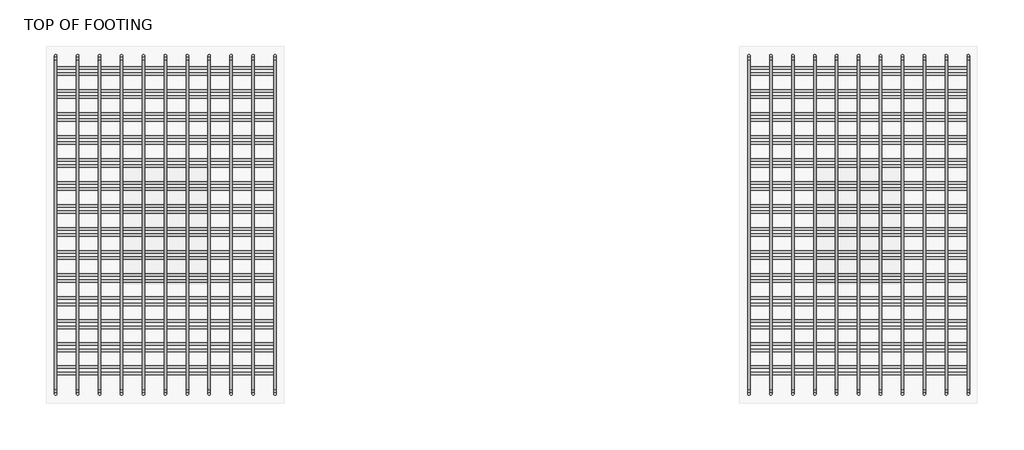
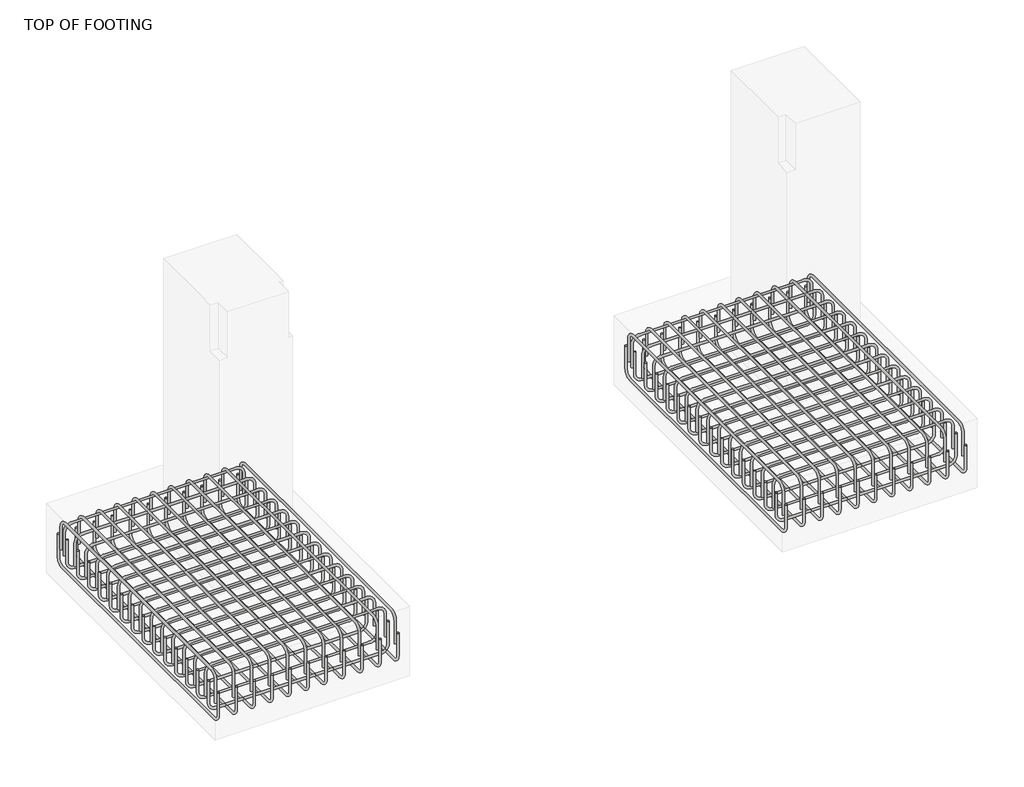
# One storey, part 11 of 11: 8 reinforcing bars.
"""IFC4 building model written with IfcOpenShell, lengths in millimetres."""

from ifc_helpers import new_model, si_unit, point, frame, origin, place, context, project, spatial, polyline, circle_curve, trimmed, segment, composite_curve, source, transform, mapped, element, save
from ifc_brep_helpers import swept_disk

model = new_model("IFC4")

# Units and contexts
model_context = context("Model", 3, world=origin())
ifc_project = project(units=[si_unit("LENGTHUNIT", "METRE", prefix="MILLI")], contexts=[model_context])

# Site, building, storey
site = spatial("IfcSite", under=ifc_project)
building = spatial("IfcBuilding", under=site)
storey = spatial("IfcBuildingStorey", under=building, Name="TOP OF FOOTING", Elevation=-1828.8)

# Reinforcing bars
placement = place(None, origin())
reinforcing_bar_shape = source(origin(), model_context, "Body", "SolidModel", [
    swept_disk(composite_curve([segment(polyline([(5183.7615906, 18549.4712443, -2012.1658531), (5183.7615906, 18549.4712443, -2159.4658531)]), True, "CONTINUOUS"), segment(trimmed(circle_curve(frame((5183.7615906, 18595.8212443, -2159.4658531), z_axis=(1.0, 0.0, 0.0), x_axis=(0.0, -46.35000000000218, 0.0)), 46.35), [point((5183.7615906, 18549.4712443, -2159.4658531))], [point((5183.7615906, 18595.8212443, -2205.8158531))], True, "CARTESIAN"), True, "CONTINUOUS"), segment(polyline([(5183.7615906, 18595.8212443, -2205.8158531), (5183.7615906, 20210.4212443, -2205.8158531)]), True, "CONTINUOUS"), segment(trimmed(circle_curve(frame((5183.7615906, 20210.4212443, -2159.4658531), z_axis=(1.0, 0.0, 0.0), x_axis=(0.0, 0.0, -46.34999999999991)), 46.35), [point((5183.7615906, 20210.4212443, -2205.8158531))], [point((5183.7615906, 20256.7712443, -2159.4658531))], True, "CARTESIAN"), True, "CONTINUOUS"), segment(polyline([(5183.7615906, 20256.7712443, -2159.4658531), (5183.7615906, 20256.7712443, -2012.1658531)]), True, "CONTINUOUS")], self_intersect=False), 6.35),
])
element("IfcReinforcingBar", 1, at=placement, inside=storey, context=model_context, shape_type="MappedRepresentation", body=[
    mapped(reinforcing_bar_shape, transform((0.0, 0.0, 0.0), x_axis=(1.0, 0.0, 0.0), y_axis=(0.0, 1.0, 0.0), z_axis=(0.0, 0.0, 1.0))),
    mapped(reinforcing_bar_shape, transform((-110.73, 0.0, 0.0), x_axis=(1.0, 0.0, 0.0), y_axis=(0.0, 1.0, 0.0), z_axis=(0.0, 0.0, 1.0))),
    mapped(reinforcing_bar_shape, transform((-221.46, 0.0, 0.0), x_axis=(1.0, 0.0, 0.0), y_axis=(0.0, 1.0, 0.0), z_axis=(0.0, 0.0, 1.0))),
    mapped(reinforcing_bar_shape, transform((-332.19, 0.0, 0.0), x_axis=(1.0, 0.0, 0.0), y_axis=(0.0, 1.0, 0.0), z_axis=(0.0, 0.0, 1.0))),
    mapped(reinforcing_bar_shape, transform((-442.92, 0.0, 0.0), x_axis=(1.0, 0.0, 0.0), y_axis=(0.0, 1.0, 0.0), z_axis=(0.0, 0.0, 1.0))),
    mapped(reinforcing_bar_shape, transform((-553.65, 0.0, 0.0), x_axis=(1.0, 0.0, 0.0), y_axis=(0.0, 1.0, 0.0), z_axis=(0.0, 0.0, 1.0))),
    mapped(reinforcing_bar_shape, transform((-664.38, 0.0, 0.0), x_axis=(1.0, 0.0, 0.0), y_axis=(0.0, 1.0, 0.0), z_axis=(0.0, 0.0, 1.0))),
    mapped(reinforcing_bar_shape, transform((-775.11, 0.0, 0.0), x_axis=(1.0, 0.0, 0.0), y_axis=(0.0, 1.0, 0.0), z_axis=(0.0, 0.0, 1.0))),
    mapped(reinforcing_bar_shape, transform((-885.84, 0.0, 0.0), x_axis=(1.0, 0.0, 0.0), y_axis=(0.0, 1.0, 0.0), z_axis=(0.0, 0.0, 1.0))),
    mapped(reinforcing_bar_shape, transform((-996.57, 0.0, 0.0), x_axis=(1.0, 0.0, 0.0), y_axis=(0.0, 1.0, 0.0), z_axis=(0.0, 0.0, 1.0))),
    mapped(reinforcing_bar_shape, transform((-1107.3, 0.0, 0.0), x_axis=(1.0, 0.0, 0.0), y_axis=(0.0, 1.0, 0.0), z_axis=(0.0, 0.0, 1.0))),
])
reinforcing_bar_2_shape = source(origin(), model_context, "Body", "SolidModel", [
    swept_disk(composite_curve([segment(polyline([(4076.4615906, 18577.6603603, -2096.8914539), (4076.4615906, 18577.6603603, -1949.5914539)]), True, "CONTINUOUS"), segment(trimmed(circle_curve(frame((4076.4615906, 18624.0103603, -1949.5914539), z_axis=(-1.0, 0.0, 0.0), x_axis=(0.0, -46.349999999998545, 0.0)), 46.35), [point((4076.4615906, 18577.6603603, -1949.5914539))], [point((4076.4615906, 18624.0103603, -1903.2414539))], True, "CARTESIAN"), True, "CONTINUOUS"), segment(polyline([(4076.4615906, 18624.0103603, -1903.2414539), (4076.4615906, 20181.3238837, -1903.2414539)]), True, "CONTINUOUS"), segment(trimmed(circle_curve(frame((4076.4615906, 20181.3238837, -1949.5914539), z_axis=(-1.0, 0.0, 0.0), x_axis=(0.0, 0.0, 46.350000000000136)), 46.35), [point((4076.4615906, 20181.3238837, -1903.2414539))], [point((4076.4615906, 20227.6738837, -1949.5914539))], True, "CARTESIAN"), True, "CONTINUOUS"), segment(polyline([(4076.4615906, 20227.6738837, -1949.5914539), (4076.4615906, 20227.6738837, -2096.8914539)]), True, "CONTINUOUS")], self_intersect=False), 6.35),
])
element("IfcReinforcingBar", 2, at=placement, inside=storey, context=model_context, shape_type="MappedRepresentation", body=[
    mapped(reinforcing_bar_2_shape, transform((0.0, 0.0, 0.0), x_axis=(1.0, 0.0, 0.0), y_axis=(0.0, 1.0, 0.0), z_axis=(0.0, 0.0, 1.0))),
    mapped(reinforcing_bar_2_shape, transform((110.73, 0.0, 0.0), x_axis=(1.0, 0.0, 0.0), y_axis=(0.0, 1.0, 0.0), z_axis=(0.0, 0.0, 1.0))),
    mapped(reinforcing_bar_2_shape, transform((221.46, 0.0, 0.0), x_axis=(1.0, 0.0, 0.0), y_axis=(0.0, 1.0, 0.0), z_axis=(0.0, 0.0, 1.0))),
    mapped(reinforcing_bar_2_shape, transform((332.19, 0.0, 0.0), x_axis=(1.0, 0.0, 0.0), y_axis=(0.0, 1.0, 0.0), z_axis=(0.0, 0.0, 1.0))),
    mapped(reinforcing_bar_2_shape, transform((442.92, 0.0, 0.0), x_axis=(1.0, 0.0, 0.0), y_axis=(0.0, 1.0, 0.0), z_axis=(0.0, 0.0, 1.0))),
    mapped(reinforcing_bar_2_shape, transform((553.65, 0.0, 0.0), x_axis=(1.0, 0.0, 0.0), y_axis=(0.0, 1.0, 0.0), z_axis=(0.0, 0.0, 1.0))),
    mapped(reinforcing_bar_2_shape, transform((664.38, 0.0, 0.0), x_axis=(1.0, 0.0, 0.0), y_axis=(0.0, 1.0, 0.0), z_axis=(0.0, 0.0, 1.0))),
    mapped(reinforcing_bar_2_shape, transform((775.11, 0.0, 0.0), x_axis=(1.0, 0.0, 0.0), y_axis=(0.0, 1.0, 0.0), z_axis=(0.0, 0.0, 1.0))),
    mapped(reinforcing_bar_2_shape, transform((885.84, 0.0, 0.0), x_axis=(1.0, 0.0, 0.0), y_axis=(0.0, 1.0, 0.0), z_axis=(0.0, 0.0, 1.0))),
    mapped(reinforcing_bar_2_shape, transform((996.57, 0.0, 0.0), x_axis=(1.0, 0.0, 0.0), y_axis=(0.0, 1.0, 0.0), z_axis=(0.0, 0.0, 1.0))),
    mapped(reinforcing_bar_2_shape, transform((1107.3, 0.0, 0.0), x_axis=(1.0, 0.0, 0.0), y_axis=(0.0, 1.0, 0.0), z_axis=(0.0, 0.0, 1.0))),
])
reinforcing_bar_3_shape = source(origin(), model_context, "Body", "SolidModel", [
    swept_disk(composite_curve([segment(polyline([(4076.4615906, 18653.1930221, -1996.7664426), (4076.4615906, 18653.1930221, -2144.0664426)]), True, "CONTINUOUS"), segment(trimmed(circle_curve(frame((4122.8115906, 18653.1930221, -2144.0664426), z_axis=(0.0, -1.0, 0.0), x_axis=(-46.350000000000364, 0.0, 0.0)), 46.35), [point((4076.4615906, 18653.1930221, -2144.0664426))], [point((4122.8115906, 18653.1930221, -2190.4164426))], True, "CARTESIAN"), True, "CONTINUOUS"), segment(polyline([(4122.8115906, 18653.1930221, -2190.4164426), (5137.4115906, 18653.1930221, -2190.4164426)]), True, "CONTINUOUS"), segment(trimmed(circle_curve(frame((5137.4115906, 18653.1930221, -2144.0664426), z_axis=(0.0, -1.0, 0.0), x_axis=(0.0, 0.0, -46.350000000000364)), 46.35), [point((5137.4115906, 18653.1930221, -2190.4164426))], [point((5183.7615906, 18653.1930221, -2144.0664426))], True, "CARTESIAN"), True, "CONTINUOUS"), segment(polyline([(5183.7615906, 18653.1930221, -2144.0664426), (5183.7615906, 18653.1930221, -1996.7664426)]), True, "CONTINUOUS")], self_intersect=False), 6.35),
])
element("IfcReinforcingBar", 3, at=placement, inside=storey, context=model_context, shape_type="MappedRepresentation", body=[
    mapped(reinforcing_bar_3_shape, transform((0.0, 0.0, 0.0), x_axis=(1.0, 0.0, 0.0), y_axis=(0.0, 1.0, 0.0), z_axis=(0.0, 0.0, 1.0))),
    mapped(reinforcing_bar_3_shape, transform((0.0, 116.2744005, 0.0), x_axis=(1.0, 0.0, 0.0), y_axis=(0.0, 1.0, 0.0), z_axis=(0.0, 0.0, 1.0))),
    mapped(reinforcing_bar_3_shape, transform((0.0, 232.5488009, 0.0), x_axis=(1.0, 0.0, 0.0), y_axis=(0.0, 1.0, 0.0), z_axis=(0.0, 0.0, 1.0))),
    mapped(reinforcing_bar_3_shape, transform((0.0, 348.8232014, 0.0), x_axis=(1.0, 0.0, 0.0), y_axis=(0.0, 1.0, 0.0), z_axis=(0.0, 0.0, 1.0))),
    mapped(reinforcing_bar_3_shape, transform((0.0, 465.0976018, 0.0), x_axis=(1.0, 0.0, 0.0), y_axis=(0.0, 1.0, 0.0), z_axis=(0.0, 0.0, 1.0))),
    mapped(reinforcing_bar_3_shape, transform((0.0, 581.3720023, 0.0), x_axis=(1.0, 0.0, 0.0), y_axis=(0.0, 1.0, 0.0), z_axis=(0.0, 0.0, 1.0))),
    mapped(reinforcing_bar_3_shape, transform((0.0, 697.6464027, 0.0), x_axis=(1.0, 0.0, 0.0), y_axis=(0.0, 1.0, 0.0), z_axis=(0.0, 0.0, 1.0))),
    mapped(reinforcing_bar_3_shape, transform((0.0, 813.9208032, 0.0), x_axis=(1.0, 0.0, 0.0), y_axis=(0.0, 1.0, 0.0), z_axis=(0.0, 0.0, 1.0))),
    mapped(reinforcing_bar_3_shape, transform((0.0, 930.1952036, 0.0), x_axis=(1.0, 0.0, 0.0), y_axis=(0.0, 1.0, 0.0), z_axis=(0.0, 0.0, 1.0))),
    mapped(reinforcing_bar_3_shape, transform((0.0, 1046.4696041, 0.0), x_axis=(1.0, 0.0, 0.0), y_axis=(0.0, 1.0, 0.0), z_axis=(0.0, 0.0, 1.0))),
    mapped(reinforcing_bar_3_shape, transform((0.0, 1162.7440045, 0.0), x_axis=(1.0, 0.0, 0.0), y_axis=(0.0, 1.0, 0.0), z_axis=(0.0, 0.0, 1.0))),
    mapped(reinforcing_bar_3_shape, transform((0.0, 1279.018405, 0.0), x_axis=(1.0, 0.0, 0.0), y_axis=(0.0, 1.0, 0.0), z_axis=(0.0, 0.0, 1.0))),
    mapped(reinforcing_bar_3_shape, transform((0.0, 1395.2928054, 0.0), x_axis=(1.0, 0.0, 0.0), y_axis=(0.0, 1.0, 0.0), z_axis=(0.0, 0.0, 1.0))),
    mapped(reinforcing_bar_3_shape, transform((0.0, 1511.5672059, 0.0), x_axis=(1.0, 0.0, 0.0), y_axis=(0.0, 1.0, 0.0), z_axis=(0.0, 0.0, 1.0))),
])
reinforcing_bar_4_shape = source(origin(), model_context, "Body", "SolidModel", [
    swept_disk(composite_curve([segment(polyline([(4076.4615906, 20194.4257435, -2114.1958609), (4076.4615906, 20194.4257435, -1966.8958609)]), True, "CONTINUOUS"), segment(trimmed(circle_curve(frame((4122.8115906, 20194.4257435, -1966.8958609), z_axis=(0.0, 1.0, 0.0), x_axis=(-46.350000000000364, 0.0, 0.0)), 46.35), [point((4076.4615906, 20194.4257435, -1966.8958609))], [point((4122.8115906, 20194.4257435, -1920.5458609))], True, "CARTESIAN"), True, "CONTINUOUS"), segment(polyline([(4122.8115906, 20194.4257435, -1920.5458609), (5137.4115906, 20194.4257435, -1920.5458609)]), True, "CONTINUOUS"), segment(trimmed(circle_curve(frame((5137.4115906, 20194.4257435, -1966.8958609), z_axis=(0.0, 1.0, 0.0), x_axis=(0.0, 0.0, 46.34999999999991)), 46.35), [point((5137.4115906, 20194.4257435, -1920.5458609))], [point((5183.7615906, 20194.4257435, -1966.8958609))], True, "CARTESIAN"), True, "CONTINUOUS"), segment(polyline([(5183.7615906, 20194.4257435, -1966.8958609), (5183.7615906, 20194.4257435, -2114.1958609)]), True, "CONTINUOUS")], self_intersect=False), 6.35),
])
element("IfcReinforcingBar", 4, at=placement, inside=storey, context=model_context, shape_type="MappedRepresentation", body=[
    mapped(reinforcing_bar_4_shape, transform((0.0, 0.0, 0.0), x_axis=(1.0, 0.0, 0.0), y_axis=(0.0, 1.0, 0.0), z_axis=(0.0, 0.0, 1.0))),
    mapped(reinforcing_bar_4_shape, transform((0.0, -116.1057918, 0.0), x_axis=(1.0, 0.0, 0.0), y_axis=(0.0, 1.0, 0.0), z_axis=(0.0, 0.0, 1.0))),
    mapped(reinforcing_bar_4_shape, transform((0.0, -232.2115836, 0.0), x_axis=(1.0, 0.0, 0.0), y_axis=(0.0, 1.0, 0.0), z_axis=(0.0, 0.0, 1.0))),
    mapped(reinforcing_bar_4_shape, transform((0.0, -348.3173754, 0.0), x_axis=(1.0, 0.0, 0.0), y_axis=(0.0, 1.0, 0.0), z_axis=(0.0, 0.0, 1.0))),
    mapped(reinforcing_bar_4_shape, transform((0.0, -464.4231672, 0.0), x_axis=(1.0, 0.0, 0.0), y_axis=(0.0, 1.0, 0.0), z_axis=(0.0, 0.0, 1.0))),
    mapped(reinforcing_bar_4_shape, transform((0.0, -580.528959, 0.0), x_axis=(1.0, 0.0, 0.0), y_axis=(0.0, 1.0, 0.0), z_axis=(0.0, 0.0, 1.0))),
    mapped(reinforcing_bar_4_shape, transform((0.0, -696.6347508, 0.0), x_axis=(1.0, 0.0, 0.0), y_axis=(0.0, 1.0, 0.0), z_axis=(0.0, 0.0, 1.0))),
    mapped(reinforcing_bar_4_shape, transform((0.0, -812.7405426, 0.0), x_axis=(1.0, 0.0, 0.0), y_axis=(0.0, 1.0, 0.0), z_axis=(0.0, 0.0, 1.0))),
    mapped(reinforcing_bar_4_shape, transform((0.0, -928.8463344, 0.0), x_axis=(1.0, 0.0, 0.0), y_axis=(0.0, 1.0, 0.0), z_axis=(0.0, 0.0, 1.0))),
    mapped(reinforcing_bar_4_shape, transform((0.0, -1044.9521262, 0.0), x_axis=(1.0, 0.0, 0.0), y_axis=(0.0, 1.0, 0.0), z_axis=(0.0, 0.0, 1.0))),
    mapped(reinforcing_bar_4_shape, transform((0.0, -1161.057918, 0.0), x_axis=(1.0, 0.0, 0.0), y_axis=(0.0, 1.0, 0.0), z_axis=(0.0, 0.0, 1.0))),
    mapped(reinforcing_bar_4_shape, transform((0.0, -1277.1637098, 0.0), x_axis=(1.0, 0.0, 0.0), y_axis=(0.0, 1.0, 0.0), z_axis=(0.0, 0.0, 1.0))),
    mapped(reinforcing_bar_4_shape, transform((0.0, -1393.2695016, 0.0), x_axis=(1.0, 0.0, 0.0), y_axis=(0.0, 1.0, 0.0), z_axis=(0.0, 0.0, 1.0))),
    mapped(reinforcing_bar_4_shape, transform((0.0, -1509.3752934, 0.0), x_axis=(1.0, 0.0, 0.0), y_axis=(0.0, 1.0, 0.0), z_axis=(0.0, 0.0, 1.0))),
])
reinforcing_bar_5_shape = source(origin(), model_context, "Body", "SolidModel", [
    swept_disk(composite_curve([segment(polyline([(8683.7615906, 18549.4712443, -2012.1658531), (8683.7615906, 18549.4712443, -2159.4658531)]), True, "CONTINUOUS"), segment(trimmed(circle_curve(frame((8683.7615906, 18595.8212443, -2159.4658531), z_axis=(1.0, 0.0, 0.0), x_axis=(0.0, -46.35000000000218, 0.0)), 46.35), [point((8683.7615906, 18549.4712443, -2159.4658531))], [point((8683.7615906, 18595.8212443, -2205.8158531))], True, "CARTESIAN"), True, "CONTINUOUS"), segment(polyline([(8683.7615906, 18595.8212443, -2205.8158531), (8683.7615906, 20210.4212443, -2205.8158531)]), True, "CONTINUOUS"), segment(trimmed(circle_curve(frame((8683.7615906, 20210.4212443, -2159.4658531), z_axis=(1.0, 0.0, 0.0), x_axis=(0.0, 0.0, -46.34999999999991)), 46.35), [point((8683.7615906, 20210.4212443, -2205.8158531))], [point((8683.7615906, 20256.7712443, -2159.4658531))], True, "CARTESIAN"), True, "CONTINUOUS"), segment(polyline([(8683.7615906, 20256.7712443, -2159.4658531), (8683.7615906, 20256.7712443, -2012.1658531)]), True, "CONTINUOUS")], self_intersect=False), 6.35),
])
element("IfcReinforcingBar", 5, at=placement, inside=storey, context=model_context, shape_type="MappedRepresentation", body=[
    mapped(reinforcing_bar_5_shape, transform((0.0, 0.0, 0.0), x_axis=(1.0, 0.0, 0.0), y_axis=(0.0, 1.0, 0.0), z_axis=(0.0, 0.0, 1.0))),
    mapped(reinforcing_bar_5_shape, transform((-110.73, 0.0, 0.0), x_axis=(1.0, 0.0, 0.0), y_axis=(0.0, 1.0, 0.0), z_axis=(0.0, 0.0, 1.0))),
    mapped(reinforcing_bar_5_shape, transform((-221.46, 0.0, 0.0), x_axis=(1.0, 0.0, 0.0), y_axis=(0.0, 1.0, 0.0), z_axis=(0.0, 0.0, 1.0))),
    mapped(reinforcing_bar_5_shape, transform((-332.19, 0.0, 0.0), x_axis=(1.0, 0.0, 0.0), y_axis=(0.0, 1.0, 0.0), z_axis=(0.0, 0.0, 1.0))),
    mapped(reinforcing_bar_5_shape, transform((-442.92, 0.0, 0.0), x_axis=(1.0, 0.0, 0.0), y_axis=(0.0, 1.0, 0.0), z_axis=(0.0, 0.0, 1.0))),
    mapped(reinforcing_bar_5_shape, transform((-553.65, 0.0, 0.0), x_axis=(1.0, 0.0, 0.0), y_axis=(0.0, 1.0, 0.0), z_axis=(0.0, 0.0, 1.0))),
    mapped(reinforcing_bar_5_shape, transform((-664.38, 0.0, 0.0), x_axis=(1.0, 0.0, 0.0), y_axis=(0.0, 1.0, 0.0), z_axis=(0.0, 0.0, 1.0))),
    mapped(reinforcing_bar_5_shape, transform((-775.11, 0.0, 0.0), x_axis=(1.0, 0.0, 0.0), y_axis=(0.0, 1.0, 0.0), z_axis=(0.0, 0.0, 1.0))),
    mapped(reinforcing_bar_5_shape, transform((-885.84, 0.0, 0.0), x_axis=(1.0, 0.0, 0.0), y_axis=(0.0, 1.0, 0.0), z_axis=(0.0, 0.0, 1.0))),
    mapped(reinforcing_bar_5_shape, transform((-996.57, 0.0, 0.0), x_axis=(1.0, 0.0, 0.0), y_axis=(0.0, 1.0, 0.0), z_axis=(0.0, 0.0, 1.0))),
    mapped(reinforcing_bar_5_shape, transform((-1107.3, 0.0, 0.0), x_axis=(1.0, 0.0, 0.0), y_axis=(0.0, 1.0, 0.0), z_axis=(0.0, 0.0, 1.0))),
])
reinforcing_bar_6_shape = source(origin(), model_context, "Body", "SolidModel", [
    swept_disk(composite_curve([segment(polyline([(7576.4615906, 18577.6603603, -2096.8914539), (7576.4615906, 18577.6603603, -1949.5914539)]), True, "CONTINUOUS"), segment(trimmed(circle_curve(frame((7576.4615906, 18624.0103603, -1949.5914539), z_axis=(-1.0, 0.0, 0.0), x_axis=(0.0, -46.349999999998545, 0.0)), 46.35), [point((7576.4615906, 18577.6603603, -1949.5914539))], [point((7576.4615906, 18624.0103603, -1903.2414539))], True, "CARTESIAN"), True, "CONTINUOUS"), segment(polyline([(7576.4615906, 18624.0103603, -1903.2414539), (7576.4615906, 20181.3238837, -1903.2414539)]), True, "CONTINUOUS"), segment(trimmed(circle_curve(frame((7576.4615906, 20181.3238837, -1949.5914539), z_axis=(-1.0, 0.0, 0.0), x_axis=(0.0, 0.0, 46.350000000000136)), 46.35), [point((7576.4615906, 20181.3238837, -1903.2414539))], [point((7576.4615906, 20227.6738837, -1949.5914539))], True, "CARTESIAN"), True, "CONTINUOUS"), segment(polyline([(7576.4615906, 20227.6738837, -1949.5914539), (7576.4615906, 20227.6738837, -2096.8914539)]), True, "CONTINUOUS")], self_intersect=False), 6.35),
])
element("IfcReinforcingBar", 6, at=placement, inside=storey, context=model_context, shape_type="MappedRepresentation", body=[
    mapped(reinforcing_bar_6_shape, transform((0.0, 0.0, 0.0), x_axis=(1.0, 0.0, 0.0), y_axis=(0.0, 1.0, 0.0), z_axis=(0.0, 0.0, 1.0))),
    mapped(reinforcing_bar_6_shape, transform((110.73, 0.0, 0.0), x_axis=(1.0, 0.0, 0.0), y_axis=(0.0, 1.0, 0.0), z_axis=(0.0, 0.0, 1.0))),
    mapped(reinforcing_bar_6_shape, transform((221.46, 0.0, 0.0), x_axis=(1.0, 0.0, 0.0), y_axis=(0.0, 1.0, 0.0), z_axis=(0.0, 0.0, 1.0))),
    mapped(reinforcing_bar_6_shape, transform((332.19, 0.0, 0.0), x_axis=(1.0, 0.0, 0.0), y_axis=(0.0, 1.0, 0.0), z_axis=(0.0, 0.0, 1.0))),
    mapped(reinforcing_bar_6_shape, transform((442.92, 0.0, 0.0), x_axis=(1.0, 0.0, 0.0), y_axis=(0.0, 1.0, 0.0), z_axis=(0.0, 0.0, 1.0))),
    mapped(reinforcing_bar_6_shape, transform((553.65, 0.0, 0.0), x_axis=(1.0, 0.0, 0.0), y_axis=(0.0, 1.0, 0.0), z_axis=(0.0, 0.0, 1.0))),
    mapped(reinforcing_bar_6_shape, transform((664.38, 0.0, 0.0), x_axis=(1.0, 0.0, 0.0), y_axis=(0.0, 1.0, 0.0), z_axis=(0.0, 0.0, 1.0))),
    mapped(reinforcing_bar_6_shape, transform((775.11, 0.0, 0.0), x_axis=(1.0, 0.0, 0.0), y_axis=(0.0, 1.0, 0.0), z_axis=(0.0, 0.0, 1.0))),
    mapped(reinforcing_bar_6_shape, transform((885.84, 0.0, 0.0), x_axis=(1.0, 0.0, 0.0), y_axis=(0.0, 1.0, 0.0), z_axis=(0.0, 0.0, 1.0))),
    mapped(reinforcing_bar_6_shape, transform((996.57, 0.0, 0.0), x_axis=(1.0, 0.0, 0.0), y_axis=(0.0, 1.0, 0.0), z_axis=(0.0, 0.0, 1.0))),
    mapped(reinforcing_bar_6_shape, transform((1107.3, 0.0, 0.0), x_axis=(1.0, 0.0, 0.0), y_axis=(0.0, 1.0, 0.0), z_axis=(0.0, 0.0, 1.0))),
])
reinforcing_bar_7_shape = source(origin(), model_context, "Body", "SolidModel", [
    swept_disk(composite_curve([segment(polyline([(7576.4615906, 18653.1930221, -1996.7664426), (7576.4615906, 18653.1930221, -2144.0664426)]), True, "CONTINUOUS"), segment(trimmed(circle_curve(frame((7622.8115906, 18653.1930221, -2144.0664426), z_axis=(0.0, -1.0, 0.0), x_axis=(-46.350000000000364, 0.0, 0.0)), 46.35), [point((7576.4615906, 18653.1930221, -2144.0664426))], [point((7622.8115906, 18653.1930221, -2190.4164426))], True, "CARTESIAN"), True, "CONTINUOUS"), segment(polyline([(7622.8115906, 18653.1930221, -2190.4164426), (8637.4115906, 18653.1930221, -2190.4164426)]), True, "CONTINUOUS"), segment(trimmed(circle_curve(frame((8637.4115906, 18653.1930221, -2144.0664426), z_axis=(0.0, -1.0, 0.0), x_axis=(0.0, 0.0, -46.350000000000364)), 46.35), [point((8637.4115906, 18653.1930221, -2190.4164426))], [point((8683.7615906, 18653.1930221, -2144.0664426))], True, "CARTESIAN"), True, "CONTINUOUS"), segment(polyline([(8683.7615906, 18653.1930221, -2144.0664426), (8683.7615906, 18653.1930221, -1996.7664426)]), True, "CONTINUOUS")], self_intersect=False), 6.35),
])
element("IfcReinforcingBar", 7, at=placement, inside=storey, context=model_context, shape_type="MappedRepresentation", body=[
    mapped(reinforcing_bar_7_shape, transform((0.0, 0.0, 0.0), x_axis=(1.0, 0.0, 0.0), y_axis=(0.0, 1.0, 0.0), z_axis=(0.0, 0.0, 1.0))),
    mapped(reinforcing_bar_7_shape, transform((0.0, 116.2744005, 0.0), x_axis=(1.0, 0.0, 0.0), y_axis=(0.0, 1.0, 0.0), z_axis=(0.0, 0.0, 1.0))),
    mapped(reinforcing_bar_7_shape, transform((0.0, 232.5488009, 0.0), x_axis=(1.0, 0.0, 0.0), y_axis=(0.0, 1.0, 0.0), z_axis=(0.0, 0.0, 1.0))),
    mapped(reinforcing_bar_7_shape, transform((0.0, 348.8232014, 0.0), x_axis=(1.0, 0.0, 0.0), y_axis=(0.0, 1.0, 0.0), z_axis=(0.0, 0.0, 1.0))),
    mapped(reinforcing_bar_7_shape, transform((0.0, 465.0976018, 0.0), x_axis=(1.0, 0.0, 0.0), y_axis=(0.0, 1.0, 0.0), z_axis=(0.0, 0.0, 1.0))),
    mapped(reinforcing_bar_7_shape, transform((0.0, 581.3720023, 0.0), x_axis=(1.0, 0.0, 0.0), y_axis=(0.0, 1.0, 0.0), z_axis=(0.0, 0.0, 1.0))),
    mapped(reinforcing_bar_7_shape, transform((0.0, 697.6464027, 0.0), x_axis=(1.0, 0.0, 0.0), y_axis=(0.0, 1.0, 0.0), z_axis=(0.0, 0.0, 1.0))),
    mapped(reinforcing_bar_7_shape, transform((0.0, 813.9208032, 0.0), x_axis=(1.0, 0.0, 0.0), y_axis=(0.0, 1.0, 0.0), z_axis=(0.0, 0.0, 1.0))),
    mapped(reinforcing_bar_7_shape, transform((0.0, 930.1952036, 0.0), x_axis=(1.0, 0.0, 0.0), y_axis=(0.0, 1.0, 0.0), z_axis=(0.0, 0.0, 1.0))),
    mapped(reinforcing_bar_7_shape, transform((0.0, 1046.4696041, 0.0), x_axis=(1.0, 0.0, 0.0), y_axis=(0.0, 1.0, 0.0), z_axis=(0.0, 0.0, 1.0))),
    mapped(reinforcing_bar_7_shape, transform((0.0, 1162.7440045, 0.0), x_axis=(1.0, 0.0, 0.0), y_axis=(0.0, 1.0, 0.0), z_axis=(0.0, 0.0, 1.0))),
    mapped(reinforcing_bar_7_shape, transform((0.0, 1279.018405, 0.0), x_axis=(1.0, 0.0, 0.0), y_axis=(0.0, 1.0, 0.0), z_axis=(0.0, 0.0, 1.0))),
    mapped(reinforcing_bar_7_shape, transform((0.0, 1395.2928054, 0.0), x_axis=(1.0, 0.0, 0.0), y_axis=(0.0, 1.0, 0.0), z_axis=(0.0, 0.0, 1.0))),
    mapped(reinforcing_bar_7_shape, transform((0.0, 1511.5672059, 0.0), x_axis=(1.0, 0.0, 0.0), y_axis=(0.0, 1.0, 0.0), z_axis=(0.0, 0.0, 1.0))),
])
reinforcing_bar_8_shape = source(origin(), model_context, "Body", "SolidModel", [
    swept_disk(composite_curve([segment(polyline([(7576.4615906, 20194.4257435, -2114.1958609), (7576.4615906, 20194.4257435, -1966.8958609)]), True, "CONTINUOUS"), segment(trimmed(circle_curve(frame((7622.8115906, 20194.4257435, -1966.8958609), z_axis=(0.0, 1.0, 0.0), x_axis=(-46.350000000000364, 0.0, 0.0)), 46.35), [point((7576.4615906, 20194.4257435, -1966.8958609))], [point((7622.8115906, 20194.4257435, -1920.5458609))], True, "CARTESIAN"), True, "CONTINUOUS"), segment(polyline([(7622.8115906, 20194.4257435, -1920.5458609), (8637.4115906, 20194.4257435, -1920.5458609)]), True, "CONTINUOUS"), segment(trimmed(circle_curve(frame((8637.4115906, 20194.4257435, -1966.8958609), z_axis=(0.0, 1.0, 0.0), x_axis=(0.0, 0.0, 46.34999999999991)), 46.35), [point((8637.4115906, 20194.4257435, -1920.5458609))], [point((8683.7615906, 20194.4257435, -1966.8958609))], True, "CARTESIAN"), True, "CONTINUOUS"), segment(polyline([(8683.7615906, 20194.4257435, -1966.8958609), (8683.7615906, 20194.4257435, -2114.1958609)]), True, "CONTINUOUS")], self_intersect=False), 6.35),
])
element("IfcReinforcingBar", 8, at=placement, inside=storey, context=model_context, shape_type="MappedRepresentation", body=[
    mapped(reinforcing_bar_8_shape, transform((0.0, 0.0, 0.0), x_axis=(1.0, 0.0, 0.0), y_axis=(0.0, 1.0, 0.0), z_axis=(0.0, 0.0, 1.0))),
    mapped(reinforcing_bar_8_shape, transform((0.0, -116.1057918, 0.0), x_axis=(1.0, 0.0, 0.0), y_axis=(0.0, 1.0, 0.0), z_axis=(0.0, 0.0, 1.0))),
    mapped(reinforcing_bar_8_shape, transform((0.0, -232.2115836, 0.0), x_axis=(1.0, 0.0, 0.0), y_axis=(0.0, 1.0, 0.0), z_axis=(0.0, 0.0, 1.0))),
    mapped(reinforcing_bar_8_shape, transform((0.0, -348.3173754, 0.0), x_axis=(1.0, 0.0, 0.0), y_axis=(0.0, 1.0, 0.0), z_axis=(0.0, 0.0, 1.0))),
    mapped(reinforcing_bar_8_shape, transform((0.0, -464.4231672, 0.0), x_axis=(1.0, 0.0, 0.0), y_axis=(0.0, 1.0, 0.0), z_axis=(0.0, 0.0, 1.0))),
    mapped(reinforcing_bar_8_shape, transform((0.0, -580.528959, 0.0), x_axis=(1.0, 0.0, 0.0), y_axis=(0.0, 1.0, 0.0), z_axis=(0.0, 0.0, 1.0))),
    mapped(reinforcing_bar_8_shape, transform((0.0, -696.6347508, 0.0), x_axis=(1.0, 0.0, 0.0), y_axis=(0.0, 1.0, 0.0), z_axis=(0.0, 0.0, 1.0))),
    mapped(reinforcing_bar_8_shape, transform((0.0, -812.7405426, 0.0), x_axis=(1.0, 0.0, 0.0), y_axis=(0.0, 1.0, 0.0), z_axis=(0.0, 0.0, 1.0))),
    mapped(reinforcing_bar_8_shape, transform((0.0, -928.8463344, 0.0), x_axis=(1.0, 0.0, 0.0), y_axis=(0.0, 1.0, 0.0), z_axis=(0.0, 0.0, 1.0))),
    mapped(reinforcing_bar_8_shape, transform((0.0, -1044.9521262, 0.0), x_axis=(1.0, 0.0, 0.0), y_axis=(0.0, 1.0, 0.0), z_axis=(0.0, 0.0, 1.0))),
    mapped(reinforcing_bar_8_shape, transform((0.0, -1161.057918, 0.0), x_axis=(1.0, 0.0, 0.0), y_axis=(0.0, 1.0, 0.0), z_axis=(0.0, 0.0, 1.0))),
    mapped(reinforcing_bar_8_shape, transform((0.0, -1277.1637098, 0.0), x_axis=(1.0, 0.0, 0.0), y_axis=(0.0, 1.0, 0.0), z_axis=(0.0, 0.0, 1.0))),
    mapped(reinforcing_bar_8_shape, transform((0.0, -1393.2695016, 0.0), x_axis=(1.0, 0.0, 0.0), y_axis=(0.0, 1.0, 0.0), z_axis=(0.0, 0.0, 1.0))),
    mapped(reinforcing_bar_8_shape, transform((0.0, -1509.3752934, 0.0), x_axis=(1.0, 0.0, 0.0), y_axis=(0.0, 1.0, 0.0), z_axis=(0.0, 0.0, 1.0))),
])

save(model, "model.ifc")

# Revit data of these elements
# Elements 1, 2, 3, 4, 5, 6, 7, 8 (IfcReinforcingBar)
#   Phase Created = New Construction
